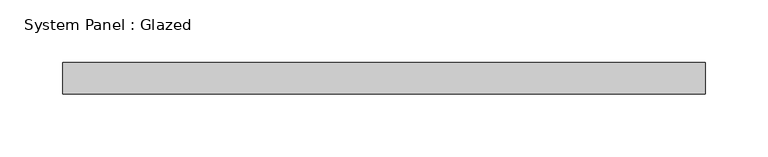
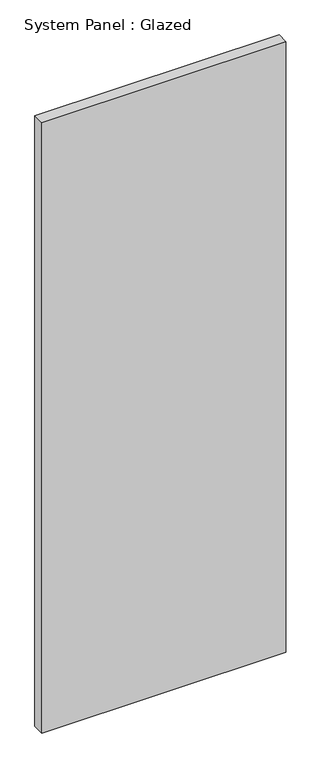
"""IFC4 building model written with IfcOpenShell, lengths in millimetres: plate geometry, System Panel : Glazed."""

from ifc_helpers import new_model, si_unit, origin, origin_with_axes, place, context, project, spatial, polyline, outline, extrude, source, transform, mapped, element, save


def system_panel_glazed_65fa7e48(model_context):
    return source(origin(), model_context, "Body", "SweptSolid", [
        extrude(outline(polyline([(257.175, 19.05), (-257.175, 19.05), (-257.175, 44.45), (257.175, 44.45), (257.175, 19.05)])), origin_with_axes(), (0.0, 0.0, 1.0), 1359.7688321),
    ])


if __name__ == "__main__":
    model = new_model("IFC4")
    model_context = context("Model", 3, world=origin())
    ifc_project = project(units=[si_unit("LENGTHUNIT", "METRE", prefix="MILLI")], contexts=[model_context])
    site = spatial("IfcSite", under=ifc_project)
    building = spatial("IfcBuilding", under=site)
    placement = place(None, origin())
    system_panel_glazed_shape = system_panel_glazed_65fa7e48(model_context)
    element("IfcPlate", 1, ObjectType="System Panel : Glazed", at=placement, inside=building, context=model_context, shape_type="MappedRepresentation", body=[
        mapped(system_panel_glazed_shape, transform((0.0, 0.0, 0.0), x_axis=(1.0, 0.0, 0.0), y_axis=(0.0, 1.0, 0.0), z_axis=(0.0, 0.0, 1.0))),
    ])
    save(model, "model.ifc")

# Revit data of these elements
# Type "System Panel : Glazed"
#   Construction Type Id = "GSP4R"
#   Analytic Construction = "1/8 in Pilkington single glazing"
#   Visual Light Transmittance = 0.9
#   Solar Heat Gain Coefficient = 0.86
#   Heat Transfer Coefficient (U) = 1.18115 BTU/(h·ft²·°F)
#   Define Thermal Properties by = 1
# Element 1 (IfcPlate, "System Panel : Glazed")
#   Materials on its faces: "Glass"
# Materials
#   "Glass": class "Glass", colour RGB 0 128 192, transparency 0.75, Description = "Soda Lime Glass", Cost = 0
